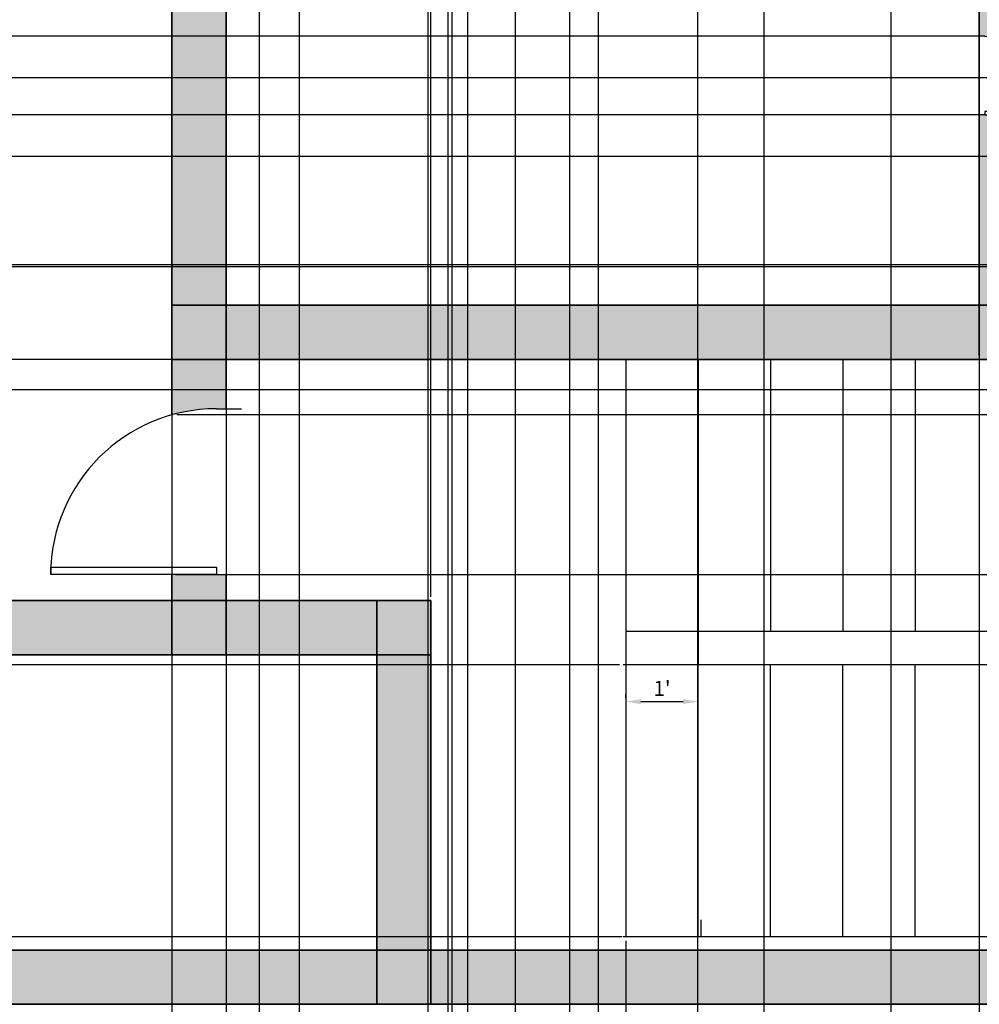
# Model space of a CAD drawing. Units: millimetres. Extents: x 2856 to 3283, y 634 to 1474.
# Tile 5 of 8: x 3006 to 3165, y 1050 to 1213. Entities that reach past the tile are written whole.
import ezdxf

# ---------------------------------------------------------------- set-up
doc = ezdxf.new("R2010")
doc.units = ezdxf.units.MM
for name, color, linetype, lineweight in [('A-ANNO-DIMS', 90, 'Continuous', 18), ('A-FLOR', 50, 'Continuous', 18), ('A-WALL-PATT', 2, 'Continuous', 13), ('doors', 10, 'Continuous', 25), ('staircase', 160, 'Continuous', 25), ('walls', 50, 'Continuous', 35)]:
    doc.layers.add(name, color=color, linetype=linetype, lineweight=lineweight)
doc.styles.get("Standard").update_dxf_attribs({"font": 'arial.ttf'})
doc.dimstyles.new('ISO-25', dxfattribs={"dimtxt": 2.5, "dimasz": 2.5, "dimexe": 1.25, "dimexo": 0.625, "dimtad": 1, "dimdec": 0, "dimlunit": 3, "dimtxsty": 'Standard', "dimcen": 2.5, "dimadec": 0, "dimazin": 0, "dimtfac": 1, "dimtdec": 0, "dimtmove": 0, "dimatfit": 3, "dimfxl": 1, "dimarcsym": 0})

# ---------------------------------------------------------------- blocks, each defined once
blk = doc.blocks.new('*D1')
at = {"layer": 'A-ANNO-DIMS', "color": 0, "lineweight": -2, "transparency": 16777216}
for p, q in [((3106.52, 1100.79), (3106.52, 1101.41)), ((3118.52, 1100.79), (3118.52, 1101.41)), ((3116.02, 1100.16), (3109.02, 1100.16))]:
    blk.add_line(p, q, dxfattribs=at)
at = {"layer": 'A-ANNO-DIMS', "color": 0, "transparency": 16777216}
for points in [[(3109.02, 1100.58), (3109.02, 1099.75), (3106.52, 1100.16)], [(3116.02, 1100.58), (3116.02, 1099.75), (3118.52, 1100.16)]]:
    blk.add_solid(points, dxfattribs=at)
at = {"layer": 'Defpoints', "color": 0, "transparency": 16777216}
for p in [(3106.52, 1100.16), (3106.52, 1100.16), (3118.52, 1100.16)]:
    blk.add_point(p, dxfattribs=at)
at = {"layer": 'A-ANNO-DIMS', "color": 0, "transparency": 16777216, "insert": (3112.52, 1102.04), "char_height": 2.5, "attachment_point": 5}
blk.add_mtext("1'", dxfattribs=at)
blk = doc.blocks.new('*U3')
for p, q in [((0, 0), (0, -6)), ((40, 0), (40, -6))]:
    blk.add_line(p, q)
blk.add_lwpolyline([(0, 0), (0, 40), (1.75, 40), (1.75, 0)], close=True)
blk.add_arc((0, 0), 40, 0, 90)
blk = doc.blocks.new('*D33')
at = {"layer": 'A-ANNO-DIMS', "color": 0, "lineweight": -2, "transparency": 16777216}
for p, q in [((3073.7, 1014.05), (3073.7, 1470.06)), ((3224.18, 1014.05), (3224.18, 1470.06)), ((3076.2, 1468.81), (3221.68, 1468.81))]:
    blk.add_line(p, q, dxfattribs=at)
at = {"layer": 'A-ANNO-DIMS', "color": 0, "transparency": 16777216}
for points in [[(3076.2, 1469.23), (3076.2, 1468.4), (3073.7, 1468.81)], [(3221.68, 1469.23), (3221.68, 1468.4), (3224.18, 1468.81)]]:
    blk.add_solid(points, dxfattribs=at)
at = {"layer": 'Defpoints', "color": 0, "transparency": 16777216}
for p in [(3224.18, 1468.81), (3073.7, 1013.42), (3224.18, 1013.42)]:
    blk.add_point(p, dxfattribs=at)
at = {"layer": 'A-ANNO-DIMS', "color": 0, "transparency": 16777216, "insert": (3148.94, 1470.73), "char_height": 2.5, "attachment_point": 5}
blk.add_mtext('12\'-6 1/2"', dxfattribs=at)
blk = doc.blocks.new('*D40')
at = {"layer": 'A-ANNO-DIMS', "color": 0, "lineweight": -2, "transparency": 16777216}
for p, q in [((3118.44, 913.07), (3118.44, 1470.06)), ((3174.82, 914.65), (3174.82, 1470.06)), ((3120.94, 1468.81), (3172.32, 1468.81))]:
    blk.add_line(p, q, dxfattribs=at)
at = {"layer": 'A-ANNO-DIMS', "color": 0, "transparency": 16777216}
for points in [[(3120.94, 1469.23), (3120.94, 1468.4), (3118.44, 1468.81)], [(3172.32, 1469.23), (3172.32, 1468.4), (3174.82, 1468.81)]]:
    blk.add_solid(points, dxfattribs=at)
at = {"layer": 'Defpoints', "color": 0, "transparency": 16777216}
for p in [(3174.82, 1468.81), (3174.82, 914.03), (3118.44, 912.44)]:
    blk.add_point(p, dxfattribs=at)
at = {"layer": 'A-ANNO-DIMS', "color": 0, "transparency": 16777216, "insert": (3146.63, 1470.73), "char_height": 2.5, "attachment_point": 5}
blk.add_mtext('4\'-8 1/2"', dxfattribs=at)
blk = doc.blocks.new('*D43')
at = {"layer": 'A-ANNO-DIMS', "color": 0, "lineweight": -2, "transparency": 16777216}
for p, q in [((3052.34, 800.56), (3052.34, 1470.06)), ((3077.68, 819.72), (3077.68, 1470.06)), ((3054.84, 1468.81), (3075.18, 1468.81))]:
    blk.add_line(p, q, dxfattribs=at)
at = {"layer": 'A-ANNO-DIMS', "color": 0, "transparency": 16777216}
for points in [[(3054.84, 1469.23), (3054.84, 1468.4), (3052.34, 1468.81)], [(3075.18, 1469.23), (3075.18, 1468.4), (3077.68, 1468.81)]]:
    blk.add_solid(points, dxfattribs=at)
at = {"layer": 'Defpoints', "color": 0, "transparency": 16777216}
for p in [(3077.68, 1468.81), (3077.68, 819.09), (3052.34, 799.94)]:
    blk.add_point(p, dxfattribs=at)
at = {"layer": 'A-ANNO-DIMS', "color": 0, "transparency": 16777216, "insert": (3065.01, 1470.73), "char_height": 2.5, "attachment_point": 5}
blk.add_mtext('2\'-1 1/2"', dxfattribs=at)
blk = doc.blocks.new('*D50')
at = {"layer": 'A-ANNO-DIMS', "color": 0, "lineweight": -2, "transparency": 16777216}
for p, q in [((3031.17, 1166.56), (3031.17, 1470.06)), ((3165.17, 1157.56), (3165.17, 1470.06)), ((3033.67, 1468.81), (3162.67, 1468.81))]:
    blk.add_line(p, q, dxfattribs=at)
at = {"layer": 'A-ANNO-DIMS', "color": 0, "transparency": 16777216}
for points in [[(3033.67, 1469.23), (3033.67, 1468.4), (3031.17, 1468.81)], [(3162.67, 1469.23), (3162.67, 1468.4), (3165.17, 1468.81)]]:
    blk.add_solid(points, dxfattribs=at)
at = {"layer": 'Defpoints', "color": 0, "transparency": 16777216}
for p in [(3165.17, 1468.81), (3031.17, 1165.94), (3165.17, 1156.94)]:
    blk.add_point(p, dxfattribs=at)
at = {"layer": 'A-ANNO-DIMS', "color": 0, "transparency": 16777216, "insert": (3098.17, 1470.69), "char_height": 2.5, "attachment_point": 5}
blk.add_mtext('11\'-2"', dxfattribs=at)
blk = doc.blocks.new('*D55')
at = {"layer": 'A-ANNO-DIMS', "color": 0, "lineweight": -2, "transparency": 16777216}
for p, q in [((3106.52, 1060.48), (3106.52, 634.81)), ((3202.52, 1060.48), (3202.52, 634.81)), ((3109.02, 636.06), (3200.02, 636.06))]:
    blk.add_line(p, q, dxfattribs=at)
at = {"layer": 'A-ANNO-DIMS', "color": 0, "transparency": 16777216}
for points in [[(3109.02, 636.48), (3109.02, 635.65), (3106.52, 636.06)], [(3200.02, 636.48), (3200.02, 635.65), (3202.52, 636.06)]]:
    blk.add_solid(points, dxfattribs=at)
at = {"layer": 'Defpoints', "color": 0, "transparency": 16777216}
for p in [(3106.52, 1061.11), (3202.52, 1061.11), (3202.52, 636.06)]:
    blk.add_point(p, dxfattribs=at)
at = {"layer": 'A-ANNO-DIMS', "color": 0, "transparency": 16777216, "insert": (3154.52, 637.96), "char_height": 2.5, "attachment_point": 5}
blk.add_mtext('8\'-0"', dxfattribs=at)
blk = doc.blocks.new('*D56')
at = {"layer": 'A-ANNO-DIMS', "color": 0, "lineweight": -2, "transparency": 16777216}
for p, q in [((3105.44, 1106.29), (2860.05, 1106.29)), ((2861.3, 1063.61), (2861.3, 1103.79)), ((3105.89, 1061.11), (2860.05, 1061.11))]:
    blk.add_line(p, q, dxfattribs=at)
at = {"layer": 'A-ANNO-DIMS', "color": 0, "transparency": 16777216}
for points in [[(2860.88, 1103.79), (2861.72, 1103.79), (2861.3, 1106.29)], [(2860.88, 1063.61), (2861.72, 1063.61), (2861.3, 1061.11)]]:
    blk.add_solid(points, dxfattribs=at)
at = {"layer": 'Defpoints', "color": 0, "transparency": 16777216}
for p in [(2861.3, 1106.29), (3106.06, 1106.29), (3106.52, 1061.11)]:
    blk.add_point(p, dxfattribs=at)
at = {"layer": 'A-ANNO-DIMS', "color": 0, "transparency": 16777216, "insert": (2859.4, 1083.7), "char_height": 2.5, "attachment_point": 5, "rotation": 90}
blk.add_mtext('3\'-9"', dxfattribs=at)
blk = doc.blocks.new('*D59')
at = {"layer": 'A-ANNO-DIMS', "color": 0, "lineweight": -2, "transparency": 16777216}
for p, q in [((2959.17, 1117.56), (2959.17, 1470.06)), ((3074.17, 1117.56), (3074.17, 1470.06)), ((2961.67, 1468.81), (3071.67, 1468.81))]:
    blk.add_line(p, q, dxfattribs=at)
at = {"layer": 'A-ANNO-DIMS', "color": 0, "transparency": 16777216}
for points in [[(2961.67, 1469.23), (2961.67, 1468.4), (2959.17, 1468.81)], [(3071.67, 1469.23), (3071.67, 1468.4), (3074.17, 1468.81)]]:
    blk.add_solid(points, dxfattribs=at)
at = {"layer": 'Defpoints', "color": 0, "transparency": 16777216}
for p in [(3074.17, 1468.81), (2959.17, 1116.94), (3074.17, 1116.94)]:
    blk.add_point(p, dxfattribs=at)
at = {"layer": 'A-ANNO-DIMS', "color": 0, "transparency": 16777216, "insert": (3016.67, 1470.71), "char_height": 2.5, "attachment_point": 5}
blk.add_mtext('9\'-7"', dxfattribs=at)
blk = doc.blocks.new('*D61')
at = {"layer": 'A-ANNO-DIMS', "color": 0, "lineweight": -2, "transparency": 16777216}
for p, q in [((3031.17, 1430.31), (3031.17, 634.81)), ((3040.17, 1430.31), (3040.17, 634.81)), ((3033.67, 636.06), (3037.67, 636.06))]:
    blk.add_line(p, q, dxfattribs=at)
at = {"layer": 'A-ANNO-DIMS', "color": 0, "transparency": 16777216}
for points in [[(3033.67, 636.48), (3033.67, 635.65), (3031.17, 636.06)], [(3037.67, 636.48), (3037.67, 635.65), (3040.17, 636.06)]]:
    blk.add_solid(points, dxfattribs=at)
at = {"layer": 'Defpoints', "color": 0, "transparency": 16777216}
for p in [(3031.17, 1430.94), (3040.17, 1430.94), (3040.17, 636.06)]:
    blk.add_point(p, dxfattribs=at)
at = {"layer": 'A-ANNO-DIMS', "color": 0, "transparency": 16777216, "insert": (3035.67, 637.96), "char_height": 2.5, "attachment_point": 5}
blk.add_mtext('0\'-9"', dxfattribs=at)
blk = doc.blocks.new('*D62')
at = {"layer": 'A-ANNO-DIMS', "color": 0, "lineweight": -2, "transparency": 16777216}
for p, q in [((3101.93, 1287.31), (3101.93, 634.81)), ((3129.44, 1287.31), (3129.44, 634.81)), ((3104.43, 636.06), (3126.94, 636.06))]:
    blk.add_line(p, q, dxfattribs=at)
at = {"layer": 'A-ANNO-DIMS', "color": 0, "transparency": 16777216}
for points in [[(3104.43, 636.48), (3104.43, 635.65), (3101.93, 636.06)], [(3126.94, 636.48), (3126.94, 635.65), (3129.44, 636.06)]]:
    blk.add_solid(points, dxfattribs=at)
at = {"layer": 'Defpoints', "color": 0, "transparency": 16777216}
for p in [(3101.93, 1287.94), (3129.44, 1287.94), (3129.44, 636.06)]:
    blk.add_point(p, dxfattribs=at)
at = {"layer": 'A-ANNO-DIMS', "color": 0, "transparency": 16777216, "insert": (3115.68, 637.98), "char_height": 2.5, "attachment_point": 5}
blk.add_mtext('2\'-3 1/2"', dxfattribs=at)
blk = doc.blocks.new('*D64')
at = {"layer": 'A-ANNO-DIMS', "color": 0, "lineweight": -2, "transparency": 16777216}
for p, q in [((3164.55, 1210.62), (2860.05, 1210.62)), ((2861.3, 1200.05), (2861.3, 1208.12)), ((3164.55, 1197.55), (2860.05, 1197.55))]:
    blk.add_line(p, q, dxfattribs=at)
at = {"layer": 'A-ANNO-DIMS', "color": 0, "transparency": 16777216}
for points in [[(2860.88, 1208.12), (2861.72, 1208.12), (2861.3, 1210.62)], [(2860.88, 1200.05), (2861.72, 1200.05), (2861.3, 1197.55)]]:
    blk.add_solid(points, dxfattribs=at)
at = {"layer": 'Defpoints', "color": 0, "transparency": 16777216}
for p in [(2861.3, 1210.62), (3165.17, 1210.62), (3165.17, 1197.55)]:
    blk.add_point(p, dxfattribs=at)
at = {"layer": 'A-ANNO-DIMS', "color": 0, "transparency": 16777216, "insert": (2859.42, 1204.09), "char_height": 2.5, "attachment_point": 5, "rotation": 90}
blk.add_mtext('1\'-1"', dxfattribs=at)
blk = doc.blocks.new('*D65')
at = {"layer": 'A-ANNO-DIMS', "color": 0, "lineweight": -2, "transparency": 16777216}
for p, q in [((3032.03, 1147.82), (3282.3, 1147.82)), ((3281.05, 1123.76), (3281.05, 1145.32)), ((3031.8, 1121.26), (3282.3, 1121.26))]:
    blk.add_line(p, q, dxfattribs=at)
at = {"layer": 'A-ANNO-DIMS', "color": 0, "transparency": 16777216}
for points in [[(3280.63, 1145.32), (3281.47, 1145.32), (3281.05, 1147.82)], [(3280.63, 1123.76), (3281.47, 1123.76), (3281.05, 1121.26)]]:
    blk.add_solid(points, dxfattribs=at)
at = {"layer": 'Defpoints', "color": 0, "transparency": 16777216}
for p in [(3031.41, 1147.82), (3281.05, 1147.82), (3031.17, 1121.26)]:
    blk.add_point(p, dxfattribs=at)
at = {"layer": 'A-ANNO-DIMS', "color": 0, "transparency": 16777216, "insert": (3279.13, 1134.54), "char_height": 2.5, "attachment_point": 5, "rotation": 90}
blk.add_mtext('2\'-2 1/2"', dxfattribs=at)
blk = doc.blocks.new('*D70')
at = {"layer": 'A-ANNO-DIMS', "color": 0, "lineweight": -2, "transparency": 16777216}
for p, q in [((3045.69, 1421.31), (3045.69, 634.81)), ((3076.97, 1421.31), (3076.97, 634.81)), ((3048.19, 636.06), (3074.47, 636.06))]:
    blk.add_line(p, q, dxfattribs=at)
at = {"layer": 'A-ANNO-DIMS', "color": 0, "transparency": 16777216}
for points in [[(3048.19, 636.48), (3048.19, 635.65), (3045.69, 636.06)], [(3074.47, 636.48), (3074.47, 635.65), (3076.97, 636.06)]]:
    blk.add_solid(points, dxfattribs=at)
at = {"layer": 'Defpoints', "color": 0, "transparency": 16777216}
for p in [(3045.69, 1421.94), (3076.97, 1421.94), (3076.97, 636.06)]:
    blk.add_point(p, dxfattribs=at)
at = {"layer": 'A-ANNO-DIMS', "color": 0, "transparency": 16777216, "insert": (3061.33, 637.98), "char_height": 2.5, "attachment_point": 5}
blk.add_mtext('2\'-7 1/2"', dxfattribs=at)
blk = doc.blocks.new('*D71')
at = {"layer": 'A-ANNO-DIMS', "color": 0, "lineweight": -2, "transparency": 16777216}
for p, q in [((3150.5, 1421.31), (3150.5, 634.81)), ((3189.65, 1421.31), (3189.65, 634.81)), ((3153, 636.06), (3187.15, 636.06))]:
    blk.add_line(p, q, dxfattribs=at)
at = {"layer": 'A-ANNO-DIMS', "color": 0, "transparency": 16777216}
for points in [[(3153, 636.48), (3153, 635.65), (3150.5, 636.06)], [(3187.15, 636.48), (3187.15, 635.65), (3189.65, 636.06)]]:
    blk.add_solid(points, dxfattribs=at)
at = {"layer": 'Defpoints', "color": 0, "transparency": 16777216}
for p in [(3150.5, 1421.94), (3189.65, 1421.94), (3189.65, 636.06)]:
    blk.add_point(p, dxfattribs=at)
at = {"layer": 'A-ANNO-DIMS', "color": 0, "transparency": 16777216, "insert": (3170.07, 637.97), "char_height": 2.5, "attachment_point": 5}
blk.add_mtext('3\'-3"', dxfattribs=at)
blk = doc.blocks.new('*D73')
at = {"layer": 'A-ANNO-DIMS', "color": 0, "lineweight": -2, "transparency": 16777216}
for p, q in [((2908.8, 1235.12), (3282.3, 1235.12)), ((3281.05, 1193.19), (3281.05, 1232.62)), ((2908.8, 1190.69), (3282.3, 1190.69))]:
    blk.add_line(p, q, dxfattribs=at)
at = {"layer": 'A-ANNO-DIMS', "color": 0, "transparency": 16777216}
for points in [[(3280.63, 1232.62), (3281.47, 1232.62), (3281.05, 1235.12)], [(3280.63, 1193.19), (3281.47, 1193.19), (3281.05, 1190.69)]]:
    blk.add_solid(points, dxfattribs=at)
at = {"layer": 'Defpoints', "color": 0, "transparency": 16777216}
for p in [(2908.17, 1235.12), (3281.05, 1235.12), (2908.17, 1190.69)]:
    blk.add_point(p, dxfattribs=at)
at = {"layer": 'A-ANNO-DIMS', "color": 0, "transparency": 16777216, "insert": (3279.13, 1212.91), "char_height": 2.5, "attachment_point": 5, "rotation": 90}
blk.add_mtext('3\'-8 1/2"', dxfattribs=at)
blk = doc.blocks.new('*D75')
at = {"layer": 'A-ANNO-DIMS', "color": 0, "lineweight": -2, "transparency": 16777216}
for p, q in [((3233.55, 1203.68), (2860.05, 1203.68)), ((2861.3, 1174.81), (2861.3, 1201.18)), ((3233.55, 1172.31), (2860.05, 1172.31))]:
    blk.add_line(p, q, dxfattribs=at)
at = {"layer": 'A-ANNO-DIMS', "color": 0, "transparency": 16777216}
for points in [[(2860.88, 1201.18), (2861.72, 1201.18), (2861.3, 1203.68)], [(2860.88, 1174.81), (2861.72, 1174.81), (2861.3, 1172.31)]]:
    blk.add_solid(points, dxfattribs=at)
at = {"layer": 'Defpoints', "color": 0, "transparency": 16777216}
for p in [(2861.3, 1203.68), (3234.17, 1203.68), (3234.17, 1172.31)]:
    blk.add_point(p, dxfattribs=at)
at = {"layer": 'A-ANNO-DIMS', "color": 0, "transparency": 16777216, "insert": (2859.38, 1188), "char_height": 2.5, "attachment_point": 5, "rotation": 90}
blk.add_mtext('2\'-7 1/2"', dxfattribs=at)
blk = doc.blocks.new('*D77')
at = {"layer": 'A-ANNO-DIMS', "color": 0, "lineweight": -2, "transparency": 16777216}
for p, q in [((3097.17, 1430.31), (3097.17, 634.81)), ((3150.5, 1421.31), (3150.5, 634.81)), ((3099.67, 636.06), (3148, 636.06))]:
    blk.add_line(p, q, dxfattribs=at)
at = {"layer": 'A-ANNO-DIMS', "color": 0, "transparency": 16777216}
for points in [[(3099.67, 636.48), (3099.67, 635.65), (3097.17, 636.06)], [(3148, 636.48), (3148, 635.65), (3150.5, 636.06)]]:
    blk.add_solid(points, dxfattribs=at)
at = {"layer": 'Defpoints', "color": 0, "transparency": 16777216}
for p in [(3097.17, 1430.94), (3150.5, 1421.94), (3150.5, 636.06)]:
    blk.add_point(p, dxfattribs=at)
at = {"layer": 'A-ANNO-DIMS', "color": 0, "transparency": 16777216, "insert": (3123.84, 637.98), "char_height": 2.5, "attachment_point": 5}
blk.add_mtext('4\'-5 1/2"', dxfattribs=at)
blk = doc.blocks.new('*D83')
at = {"layer": 'A-ANNO-DIMS', "color": 0, "lineweight": -2, "transparency": 16777216}
for p, q in [((2951.21, 1172.73), (3282.3, 1172.73)), ((3281.05, 1154.47), (3281.05, 1170.23)), ((2951.21, 1151.97), (3282.3, 1151.97))]:
    blk.add_line(p, q, dxfattribs=at)
at = {"layer": 'A-ANNO-DIMS', "color": 0, "transparency": 16777216}
for points in [[(3280.63, 1170.23), (3281.47, 1170.23), (3281.05, 1172.73)], [(3280.63, 1154.47), (3281.47, 1154.47), (3281.05, 1151.97)]]:
    blk.add_solid(points, dxfattribs=at)
at = {"layer": 'Defpoints', "color": 0, "transparency": 16777216}
for p in [(2950.58, 1172.73), (3281.05, 1172.73), (2950.58, 1151.97)]:
    blk.add_point(p, dxfattribs=at)
at = {"layer": 'A-ANNO-DIMS', "color": 0, "transparency": 16777216, "insert": (3279.15, 1162.35), "char_height": 2.5, "attachment_point": 5, "rotation": 90}
blk.add_mtext('1\'-9"', dxfattribs=at)
blk = doc.blocks.new('*D85')
at = {"layer": 'A-ANNO-DIMS', "color": 0, "lineweight": -2, "transparency": 16777216}
for p, q in [((3164.55, 1197.55), (2860.05, 1197.55)), ((2861.3, 1159.44), (2861.3, 1195.05)), ((3164.55, 1156.94), (2860.05, 1156.94))]:
    blk.add_line(p, q, dxfattribs=at)
at = {"layer": 'A-ANNO-DIMS', "color": 0, "transparency": 16777216}
for points in [[(2860.88, 1195.05), (2861.72, 1195.05), (2861.3, 1197.55)], [(2860.88, 1159.44), (2861.72, 1159.44), (2861.3, 1156.94)]]:
    blk.add_solid(points, dxfattribs=at)
at = {"layer": 'Defpoints', "color": 0, "transparency": 16777216}
for p in [(2861.3, 1197.55), (3165.17, 1197.55), (3165.17, 1156.94)]:
    blk.add_point(p, dxfattribs=at)
at = {"layer": 'A-ANNO-DIMS', "color": 0, "transparency": 16777216, "insert": (2859.38, 1177.24), "char_height": 2.5, "attachment_point": 5, "rotation": 90}
blk.add_mtext('3\'-4 1/2"', dxfattribs=at)
blk = doc.blocks.new('*D88')
at = {"layer": 'A-ANNO-DIMS', "color": 0, "lineweight": -2, "transparency": 16777216}
for p, q in [((3129.44, 1287.31), (3129.44, 634.81)), ((3165.17, 1287.31), (3165.17, 634.81)), ((3131.94, 636.06), (3162.67, 636.06))]:
    blk.add_line(p, q, dxfattribs=at)
at = {"layer": 'A-ANNO-DIMS', "color": 0, "transparency": 16777216}
for points in [[(3131.94, 636.48), (3131.94, 635.65), (3129.44, 636.06)], [(3162.67, 636.48), (3162.67, 635.65), (3165.17, 636.06)]]:
    blk.add_solid(points, dxfattribs=at)
at = {"layer": 'Defpoints', "color": 0, "transparency": 16777216}
for p in [(3129.44, 1287.94), (3165.17, 1287.94), (3165.17, 636.06)]:
    blk.add_point(p, dxfattribs=at)
at = {"layer": 'A-ANNO-DIMS', "color": 0, "transparency": 16777216, "insert": (3147.31, 637.98), "char_height": 2.5, "attachment_point": 5}
blk.add_mtext('2\'-11 1/2"', dxfattribs=at)
blk = doc.blocks.new('*D89')
at = {"layer": 'A-ANNO-DIMS', "color": 0, "lineweight": -2, "transparency": 16777216}
for p, q in [((3031.8, 1165.94), (3282.3, 1165.94)), ((3281.05, 1150.32), (3281.05, 1163.44)), ((3032.03, 1147.82), (3282.3, 1147.82))]:
    blk.add_line(p, q, dxfattribs=at)
at = {"layer": 'A-ANNO-DIMS', "color": 0, "transparency": 16777216}
for points in [[(3280.63, 1163.44), (3281.47, 1163.44), (3281.05, 1165.94)], [(3280.63, 1150.32), (3281.47, 1150.32), (3281.05, 1147.82)]]:
    blk.add_solid(points, dxfattribs=at)
at = {"layer": 'Defpoints', "color": 0, "transparency": 16777216}
for p in [(3031.17, 1165.94), (3281.05, 1165.94), (3031.41, 1147.82)]:
    blk.add_point(p, dxfattribs=at)
at = {"layer": 'A-ANNO-DIMS', "color": 0, "transparency": 16777216, "insert": (3279.15, 1156.88), "char_height": 2.5, "attachment_point": 5, "rotation": 90}
blk.add_mtext('1\'-6"', dxfattribs=at)
blk = doc.blocks.new('*D94')
at = {"layer": 'A-ANNO-DIMS', "color": 0, "lineweight": -2, "transparency": 16777216}
for p, q in [((3040.17, 1287.31), (3040.17, 634.81)), ((3080.25, 1257.69), (3080.25, 634.81)), ((3042.67, 636.06), (3077.75, 636.06))]:
    blk.add_line(p, q, dxfattribs=at)
at = {"layer": 'A-ANNO-DIMS', "color": 0, "transparency": 16777216}
for points in [[(3042.67, 636.48), (3042.67, 635.65), (3040.17, 636.06)], [(3077.75, 636.48), (3077.75, 635.65), (3080.25, 636.06)]]:
    blk.add_solid(points, dxfattribs=at)
at = {"layer": 'Defpoints', "color": 0, "transparency": 16777216}
for p in [(3040.17, 1287.94), (3080.25, 1258.32), (3080.25, 636.06)]:
    blk.add_point(p, dxfattribs=at)
at = {"layer": 'A-ANNO-DIMS', "color": 0, "transparency": 16777216, "insert": (3060.21, 637.97), "char_height": 2.5, "attachment_point": 5}
blk.add_mtext('3\'-4"', dxfattribs=at)
blk = doc.blocks.new('*D95')
at = {"layer": 'A-ANNO-DIMS', "color": 0, "lineweight": -2, "transparency": 16777216}
for p, q in [((3108.57, 1243.09), (2860.05, 1243.09)), ((2861.3, 1159.44), (2861.3, 1240.59)), ((3164.55, 1156.94), (2860.05, 1156.94))]:
    blk.add_line(p, q, dxfattribs=at)
at = {"layer": 'A-ANNO-DIMS', "color": 0, "transparency": 16777216}
for points in [[(2860.88, 1240.59), (2861.72, 1240.59), (2861.3, 1243.09)], [(2860.88, 1159.44), (2861.72, 1159.44), (2861.3, 1156.94)]]:
    blk.add_solid(points, dxfattribs=at)
at = {"layer": 'Defpoints', "color": 0, "transparency": 16777216}
for p in [(2861.3, 1243.09), (3109.2, 1243.09), (3165.17, 1156.94)]:
    blk.add_point(p, dxfattribs=at)
at = {"layer": 'A-ANNO-DIMS', "color": 0, "transparency": 16777216, "insert": (2859.42, 1200.02), "char_height": 2.5, "attachment_point": 5, "rotation": 90}
blk.add_mtext('7\'-2"', dxfattribs=at)
blk = doc.blocks.new('*D98')
at = {"layer": 'A-ANNO-DIMS', "color": 0, "lineweight": -2, "transparency": 16777216}
for p, q in [((3088.17, 1430.31), (3088.17, 634.81)), ((3076.97, 1421.31), (3076.97, 634.81)), ((3079.47, 636.06), (3085.67, 636.06))]:
    blk.add_line(p, q, dxfattribs=at)
at = {"layer": 'A-ANNO-DIMS', "color": 0, "transparency": 16777216}
for points in [[(3079.47, 636.48), (3079.47, 635.65), (3076.97, 636.06)], [(3085.67, 636.48), (3085.67, 635.65), (3088.17, 636.06)]]:
    blk.add_solid(points, dxfattribs=at)
at = {"layer": 'Defpoints', "color": 0, "transparency": 16777216}
for p in [(3088.17, 1430.94), (3076.97, 1421.94), (3088.17, 636.06)]:
    blk.add_point(p, dxfattribs=at)
at = {"layer": 'A-ANNO-DIMS', "color": 0, "transparency": 16777216, "insert": (3082.57, 637.96), "char_height": 2.5, "attachment_point": 5}
blk.add_mtext('0\'-11"', dxfattribs=at)

msp = doc.modelspace()

# ---------------------------------------------------------------- hatches: boundary and pattern name
at = {"layer": 'A-WALL-PATT'}
h = msp.add_hatch(color=256, dxfattribs=at)
h.dxf.hatch_style = 1
h.paths.add_polyline_path([(2908.17, 1430.94), (2899.17, 1430.94), (2899.17, 1421.94), (2908.17, 1421.94)])
h.paths.add_polyline_path([(2908.17, 1421.94), (2899.17, 1421.94), (2899.17, 1296.94), (2908.17, 1296.94)])
h.paths.add_polyline_path([(2940.27, 1430.94), (2908.17, 1430.94), (2908.17, 1421.94), (2940.27, 1421.94)])
h.paths.add_polyline_path([(3031.17, 1430.94), (2982.35, 1430.94), (2982.35, 1421.94), (3031.17, 1421.94)])
h.paths.add_polyline_path([(3150.5, 1430.94), (3097.17, 1430.94), (3097.17, 1421.94), (3150.5, 1421.94)])
h.paths.add_polyline_path([(3097.17, 1430.94), (3088.17, 1430.94), (3088.17, 1421.94), (3097.17, 1421.94)])
h.paths.add_polyline_path([(3097.17, 1421.94), (3088.17, 1421.94), (3088.17, 1337.94), (3097.17, 1337.94)])
h.paths.add_polyline_path([(3088.17, 1337.94), (3040.17, 1337.94), (3040.17, 1328.94), (3088.17, 1328.94)])
h.paths.add_polyline_path([(3097.17, 1337.94), (3088.17, 1337.94), (3088.17, 1328.94), (3097.17, 1328.94)])
h.paths.add_polyline_path([(3097.17, 1328.94), (3088.17, 1328.94), (3088.17, 1296.94), (3097.17, 1296.94)])
h.paths.add_polyline_path([(3097.17, 1296.94), (3088.17, 1296.94), (3088.17, 1287.94), (3097.17, 1287.94)])
h.paths.add_polyline_path([(3040.17, 1421.94), (3031.17, 1421.94), (3031.17, 1337.94), (3040.17, 1337.94)])
h.paths.add_polyline_path([(3040.17, 1337.94), (3031.17, 1337.94), (3031.17, 1328.94), (3040.17, 1328.94)])
h.paths.add_polyline_path([(3040.17, 1430.94), (3031.17, 1430.94), (3031.17, 1421.94), (3040.17, 1421.94)])
h.paths.add_polyline_path([(3243.17, 1421.94), (3234.17, 1421.94), (3234.17, 1385.21), (3243.17, 1385.21)])
h.paths.add_polyline_path([(3243.17, 1430.94), (3234.17, 1430.94), (3234.17, 1421.94), (3243.17, 1421.94)])
h.paths.add_polyline_path([(3234.17, 1430.94), (3189.65, 1430.94), (3189.65, 1421.94), (3234.17, 1421.94)])
h.paths.add_polyline_path([(3243.17, 1345.16), (3234.17, 1345.16), (3234.17, 1296.94), (3243.17, 1296.94)])
h.paths.add_polyline_path([(3234.17, 1296.94), (3128.45, 1296.94, -0.06768), (3129.44, 1289.59), (3129.44, 1287.94), (3234.17, 1287.94)])
h.paths.add_polyline_path([(3031.17, 1296.94), (2908.17, 1296.94), (2908.17, 1287.94), (3031.17, 1287.94)])
h.paths.add_polyline_path([(3040.17, 1296.94), (3031.17, 1296.94), (3031.17, 1287.94), (3040.17, 1287.94)])
h.paths.add_polyline_path([(2908.17, 1296.94), (2899.17, 1296.94), (2899.17, 1287.94), (2908.17, 1287.94)])
h.paths.add_polyline_path([(2908.17, 1287.94), (2899.17, 1287.94), (2899.17, 1235.12), (2908.17, 1235.12)])
h.paths.add_polyline_path([(3040.17, 1287.94), (3031.17, 1287.94), (3031.17, 1165.94), (3040.17, 1165.94)])
h.paths.add_polyline_path([(3165.17, 1165.94), (3040.17, 1165.94), (3040.17, 1156.94), (3165.17, 1156.94)])
h.paths.add_polyline_path([(3040.17, 1165.94), (3031.17, 1165.94), (3031.17, 1156.94), (3040.17, 1156.94)])
h.paths.add_polyline_path([(3040.17, 1156.94), (3031.17, 1156.94), (3031.17, 1147.75, -0.068303), (3038.59, 1148.77), (3040.17, 1148.77)])
h.paths.add_polyline_path([(3174.17, 1197.55), (3166.11, 1197.55), (3165.17, 1197.55), (3165.17, 1165.94), (3174.17, 1165.94)])
h.paths.add_polyline_path([(3174.17, 1165.94), (3165.17, 1165.94), (3165.17, 1156.94), (3174.17, 1156.94)])
h.paths.add_polyline_path([(3234.17, 1165.94), (3174.17, 1165.94), (3174.17, 1156.94), (3234.17, 1156.94)])
h.paths.add_polyline_path([(3243.17, 1165.94), (3234.17, 1165.94), (3234.17, 1156.94), (3243.17, 1156.94)])
h.paths.add_polyline_path([(3243.17, 1172.31), (3234.17, 1172.31), (3234.17, 1165.94), (3243.17, 1165.94)])
h.paths.add_polyline_path([(3243.17, 1222.94), (3234.17, 1222.94), (3234.17, 1213.94), (3243.17, 1213.94)])
h.paths.add_polyline_path([(3234.17, 1222.94), (3174.17, 1222.94), (3174.17, 1213.94), (3234.17, 1213.94)])
h.paths.add_polyline_path([(3174.17, 1222.94), (3165.17, 1222.94), (3165.17, 1213.94), (3174.17, 1213.94)])
h.paths.add_polyline_path([(3174.17, 1270.54, -0.139319), (3166.75, 1268.43), (3165.17, 1268.43), (3165.17, 1222.94), (3174.17, 1222.94)])
h.paths.add_polyline_path([(3243.17, 1243.94), (3234.17, 1243.94), (3234.17, 1222.94), (3243.17, 1222.94)])
h.paths.add_polyline_path([(3243.17, 1213.94), (3234.17, 1213.94), (3234.17, 1203.68), (3243.17, 1203.68)])
h.paths.add_polyline_path([(3174.17, 1213.94), (3165.17, 1213.94), (3165.17, 1210.62), (3166.11, 1210.62, -0.16772), (3174.17, 1207.84)])
h.paths.add_polyline_path([(3243.17, 1296.94), (3234.17, 1296.94), (3234.17, 1287.94), (3243.17, 1287.94)])
h.paths.add_polyline_path([(3243.17, 1287.94), (3234.17, 1287.94), (3234.17, 1276.76), (3243.17, 1276.76)])
h.paths.add_polyline_path([(3174.17, 1287.94), (3165.17, 1287.94), (3165.17, 1282.56), (3166.75, 1282.56), (3174.17, 1282.56)])
h.paths.add_polyline_path([(2908.17, 1190.69), (2899.17, 1190.69), (2899.17, 1116.94), (2908.17, 1116.94)])
h.paths.add_polyline_path([(2908.17, 1107.94), (2899.17, 1107.94), (2899.17, 1058.94), (2908.17, 1058.94)])
h.paths.add_polyline_path([(2908.17, 1116.94), (2899.17, 1116.94), (2899.17, 1107.94), (2908.17, 1107.94)])
h.paths.add_polyline_path([(2959.17, 1107.94), (2950.17, 1107.94), (2950.17, 1058.94), (2959.17, 1058.94)])
h.paths.add_polyline_path([(2959.17, 1116.94), (2950.17, 1116.94), (2950.17, 1107.94), (2959.17, 1107.94)])
h.paths.add_polyline_path([(2950.17, 1116.94), (2908.17, 1116.94), (2908.17, 1107.94), (2950.17, 1107.94)])
h.paths.add_polyline_path([(3031.17, 1116.94), (2959.17, 1116.94), (2959.17, 1107.94), (3031.17, 1107.94)])
h.paths.add_polyline_path([(3074.17, 1116.94), (3065.17, 1116.94), (3065.17, 1107.94), (3074.17, 1107.94)])
h.paths.add_polyline_path([(3065.17, 1116.94), (3040.17, 1116.94), (3040.17, 1107.94), (3065.17, 1107.94)])
h.paths.add_polyline_path([(3040.17, 1116.94), (3031.17, 1116.94), (3031.17, 1107.94), (3040.17, 1107.94)])
h.paths.add_polyline_path([(3040.17, 1121.26), (3038.59, 1121.26), (3031.17, 1121.26), (3031.17, 1116.94), (3040.17, 1116.94)])
h.paths.add_polyline_path([(3074.17, 1107.94), (3065.17, 1107.94), (3065.17, 1058.94), (3074.17, 1058.94)])
h.paths.add_polyline_path([(3074.17, 1058.94), (3065.17, 1058.94), (3065.17, 1049.94), (3074.17, 1049.94)])
h.paths.add_polyline_path([(3065.17, 1058.94), (2975.4, 1058.94, -0.174756), (2978.69, 1049.94), (3065.17, 1049.94)])
h.paths.add_polyline_path([(2929.83, 1051.89), (2930.25, 1058.94), (2908.17, 1058.94), (2908.17, 1049.94), (2929.71, 1049.94)])
h.paths.add_polyline_path([(2908.17, 1058.94), (2899.17, 1058.94), (2899.17, 1049.94), (2908.17, 1049.94)])
h.paths.add_polyline_path([(2950.17, 1058.94), (2942.07, 1058.94, -0.146602), (2943.93, 1051.05), (2943.86, 1049.94), (2950.17, 1049.94)])
h.paths.add_polyline_path([(2959.17, 1058.94), (2950.17, 1058.94), (2950.17, 1049.94), (2959.17, 1049.94)])
h.paths.add_polyline_path([(2964.56, 1058.94), (2959.17, 1058.94), (2959.17, 1049.94), (2964.56, 1049.94)])
h.paths.add_polyline_path([(2908.17, 1049.94), (2899.17, 1049.94), (2899.17, 799.94), (2908.17, 799.94)])
h.paths.add_polyline_path([(3234.17, 1058.94), (3074.17, 1058.94), (3074.17, 1049.94), (3234.17, 1049.94)])
h.paths.add_polyline_path([(3243.17, 1156.94), (3234.17, 1156.94), (3234.17, 1058.94), (3243.17, 1058.94)])
h.paths.add_polyline_path([(3243.17, 1058.94), (3234.17, 1058.94), (3234.17, 1049.94), (3243.17, 1049.94)])
h.paths.add_polyline_path([(3243.17, 1049.94), (3234.17, 1049.94), (3234.17, 931.7), (3234.17, 799.94), (3243.17, 799.94), (3243.17, 931.7)])
h.paths.add_polyline_path([(2908.17, 790.94), (2899.17, 790.94), (2899.17, 682.94), (2908.17, 682.94)])
h.paths.add_polyline_path([(2908.17, 799.94), (2899.17, 799.94), (2899.17, 790.94), (2908.17, 790.94)])
h.paths.add_polyline_path([(3234.17, 799.94), (2908.17, 799.94), (2908.17, 790.94), (3234.17, 790.94)])
h.paths.add_polyline_path([(3243.17, 799.94), (3234.17, 799.94), (3234.17, 790.94), (3243.17, 790.94)])
h.paths.add_polyline_path([(3243.17, 790.94), (3234.17, 790.94), (3234.17, 682.94), (3243.17, 682.94)])
h.paths.add_polyline_path([(3234.17, 682.94), (2908.17, 682.94), (2908.17, 673.94), (3234.17, 673.94)])
h.paths.add_polyline_path([(3243.17, 682.94), (3234.17, 682.94), (3234.17, 673.94), (3243.17, 673.94)])
h.paths.add_polyline_path([(2908.17, 682.94), (2899.17, 682.94), (2899.17, 673.94), (2908.17, 673.94)])

# ---------------------------------------------------------------- linework, layer by layer
at = {"layer": 'A-FLOR'}
msp.add_line((3052.34, 1049.94), (3052.34, 799.94), dxfattribs=at)
at = {"layer": 'staircase'}
for p, q in [((3106.52, 1156.94), (3106.52, 1061.11)), ((3118.52, 1156.94), (3118.52, 1106.29)), ((3130.52, 1156.94), (3130.52, 1111.85)), ((3142.52, 1156.94), (3142.52, 1111.85)), ((3154.52, 1156.94), (3154.52, 1111.85)), ((3106.52, 1111.85), (3202.52, 1111.85)), ((3202.52, 1106.29), (3106.06, 1106.29)), ((3118.52, 1061.11), (3118.52, 1106.29)), ((3130.52, 1061.11), (3130.52, 1106.29)), ((3142.52, 1061.11), (3142.52, 1106.29)), ((3154.52, 1061.11), (3154.52, 1106.29)), ((3118.97, 1063.94), (3118.97, 1061.11)), ((3202.52, 1061.11), (3106.06, 1061.11))]:
    msp.add_line(p, q, dxfattribs=at)
at = {"layer": 'walls'}
for p, q in [((3031.17, 1299.78), (3031.17, 1147.75)), ((3040.17, 1299.78), (3040.17, 1148.77)), ((3031.17, 1165.94), (3243.17, 1165.94)), ((3031.17, 1156.94), (3243.17, 1156.94)), ((3031.17, 1121.26), (3031.17, 1107.94)), ((3040.17, 1121.26), (3040.17, 1107.94)), ((2899.17, 1116.94), (3074.17, 1116.94)), ((3065.17, 1116.94), (3065.17, 1049.94)), ((3074.17, 1116.94), (3074.17, 1049.94)), ((2899.17, 1107.94), (3074.17, 1107.94)), ((2975.4, 1058.94), (3243.17, 1058.94)), ((2978.69, 1049.94), (3243.17, 1049.94))]:
    msp.add_line(p, q, dxfattribs=at)

# ---------------------------------------------------------------- block references
at = {"layer": 'doors'}
for p, xscale, yscale, zscale, rotation in [((3166.11, 1197.55), -0.3267993458683955, 0.3267993458683955, 0.3267993458683955, 270), ((3038.59, 1121.26), 0.6877590013859352, 0.6877590013859352, 0.6877590013859352, 90)]:
    msp.add_blockref('*U3', p, dxfattribs=dict(at, xscale=xscale, yscale=yscale, zscale=zscale, rotation=rotation))

# ---------------------------------------------------------------- dimensions: what is measured, and where the dimension line sits
at = {"layer": 'A-ANNO-DIMS'}
for base, p1, p2, override, picture, middle in [((3077.68, 1468.81), (3052.34, 799.94), (3077.68, 819.09), {"dimdec": 1, "dimlfac": 1, "dimrnd": 0, "dimzin": 1, "dimdsep": 46, "dimlunit": 4, "dimfrac": 2}, '*D43', (3065.01, 1470.73)), ((3224.18, 1468.81), (3073.7, 1013.42), (3224.18, 1013.42), {"dimdec": 1, "dimlfac": 1, "dimrnd": 0, "dimzin": 1, "dimdsep": 46, "dimlunit": 4, "dimfrac": 2}, '*D33', (3148.94, 1470.73)), ((3174.82, 1468.81), (3118.44, 912.44), (3174.82, 914.03), {"dimdec": 1, "dimlfac": 1, "dimrnd": 0, "dimzin": 1, "dimdsep": 46, "dimlunit": 4, "dimfrac": 2}, '*D40', (3146.63, 1470.73)), ((3074.17, 1468.81), (2959.17, 1116.94), (3074.17, 1116.94), {"dimdec": 1, "dimlfac": 1, "dimrnd": 0, "dimzin": 1, "dimdsep": 46, "dimlunit": 4, "dimfrac": 2}, '*D59', (3016.67, 1470.71)), ((3165.17, 1468.81), (3031.17, 1165.94), (3165.17, 1156.94), {"dimdec": 1, "dimlfac": 1, "dimrnd": 0, "dimzin": 1, "dimdsep": 46, "dimlunit": 4, "dimfrac": 2}, '*D50', (3098.17, 1470.69)), ((3040.17, 636.06), (3031.17, 1430.94), (3040.17, 1430.94), {"dimdec": 1, "dimlfac": 1, "dimrnd": 0, "dimzin": 1, "dimdsep": 46, "dimlunit": 4, "dimfrac": 2}, '*D61', (3035.67, 637.96)), ((3088.17, 636.06), (3076.97, 1421.94), (3088.17, 1430.94), {"dimdec": 1, "dimlfac": 1, "dimrnd": 0, "dimzin": 1, "dimdsep": 46, "dimlunit": 4, "dimfrac": 2}, '*D98', (3082.57, 637.96)), ((3150.5, 636.06), (3097.17, 1430.94), (3150.5, 1421.94), {"dimdec": 1, "dimlfac": 1, "dimrnd": 0, "dimzin": 1, "dimdsep": 46, "dimlunit": 4, "dimfrac": 2}, '*D77', (3123.84, 637.98)), ((3076.97, 636.06), (3045.69, 1421.94), (3076.97, 1421.94), {"dimdec": 1, "dimlfac": 1, "dimrnd": 0, "dimzin": 1, "dimdsep": 46, "dimlunit": 4, "dimfrac": 2}, '*D70', (3061.33, 637.98)), ((3189.6495, 636.0634), (3150.4985, 1421.9396), (3189.6495, 1421.9396), {"dimdec": 1, "dimlfac": 1, "dimrnd": 0, "dimzin": 1, "dimdsep": 46, "dimlunit": 4, "dimfrac": 2}, '*D71', (3170.074, 637.9657)), ((3080.25, 636.06), (3040.17, 1287.94), (3080.25, 1258.32), {"dimdec": 1, "dimlfac": 1, "dimrnd": 0, "dimzin": 1, "dimdsep": 46, "dimlunit": 4, "dimfrac": 2}, '*D94', (3060.21, 637.97)), ((3129.44, 636.06), (3101.93, 1287.94), (3129.44, 1287.94), {"dimdec": 1, "dimlfac": 1, "dimrnd": 0, "dimzin": 1, "dimdsep": 46, "dimlunit": 4, "dimfrac": 2}, '*D62', (3115.68, 637.98)), ((3165.17, 636.06), (3129.44, 1287.94), (3165.17, 1287.94), {"dimdec": 1, "dimlfac": 1, "dimrnd": 0, "dimzin": 1, "dimdsep": 46, "dimlunit": 4, "dimfrac": 2}, '*D88', (3147.31, 637.98)), ((3106.52, 1100.16), (3118.52, 1100.16), (3106.52, 1100.16), {"dimclrd": 0, "dimclre": 0, "dimclrt": 0}, '*D1', (3112.52, 1102.04)), ((3202.52, 636.06), (3106.52, 1061.11), (3202.52, 1061.11), {"dimdec": 1, "dimlfac": 1, "dimrnd": 0, "dimzin": 1, "dimdsep": 46, "dimlunit": 4, "dimfrac": 2}, '*D55', (3154.52, 637.96))]:
    dim = msp.add_linear_dim(base=base, p1=p1, p2=p2, dimstyle='ISO-25', override=override, dxfattribs=at)
    dim.commit()
    dim.dimension.update_dxf_attribs({"geometry": picture, "text_midpoint": middle})
for base, p1, p2, picture, middle in [((2861.3003, 1243.0939), (3165.1743, 1156.9396), (3109.1985, 1243.0939), '*D95', (2859.4202, 1200.0167)), ((3281.05, 1235.12), (2908.17, 1190.69), (2908.17, 1235.12), '*D73', (3279.13, 1212.91)), ((2861.3, 1210.62), (3165.17, 1197.55), (3165.17, 1210.62), '*D64', (2859.42, 1204.09)), ((2861.3, 1203.68), (3234.17, 1172.31), (3234.17, 1203.68), '*D75', (2859.38, 1188)), ((2861.3, 1197.55), (3165.17, 1156.94), (3165.17, 1197.55), '*D85', (2859.38, 1177.24)), ((3281.05, 1172.73), (2950.58, 1151.97), (2950.58, 1172.73), '*D83', (3279.15, 1162.35)), ((3281.05, 1165.94), (3031.41, 1147.82), (3031.17, 1165.94), '*D89', (3279.15, 1156.88)), ((3281.05, 1147.82), (3031.17, 1121.26), (3031.41, 1147.82), '*D65', (3279.13, 1134.54)), ((2861.3, 1106.29), (3106.52, 1061.11), (3106.06, 1106.29), '*D56', (2859.4, 1083.7))]:
    dim = msp.add_linear_dim(base=base, p1=p1, p2=p2, angle=90, dimstyle='ISO-25', override={"dimdec": 1, "dimlfac": 1, "dimrnd": 0, "dimzin": 1, "dimdsep": 46, "dimlunit": 4, "dimfrac": 2}, dxfattribs=at)
    dim.commit()
    dim.dimension.update_dxf_attribs({"geometry": picture, "text_midpoint": middle})

doc.saveas('drawing.dxf')
